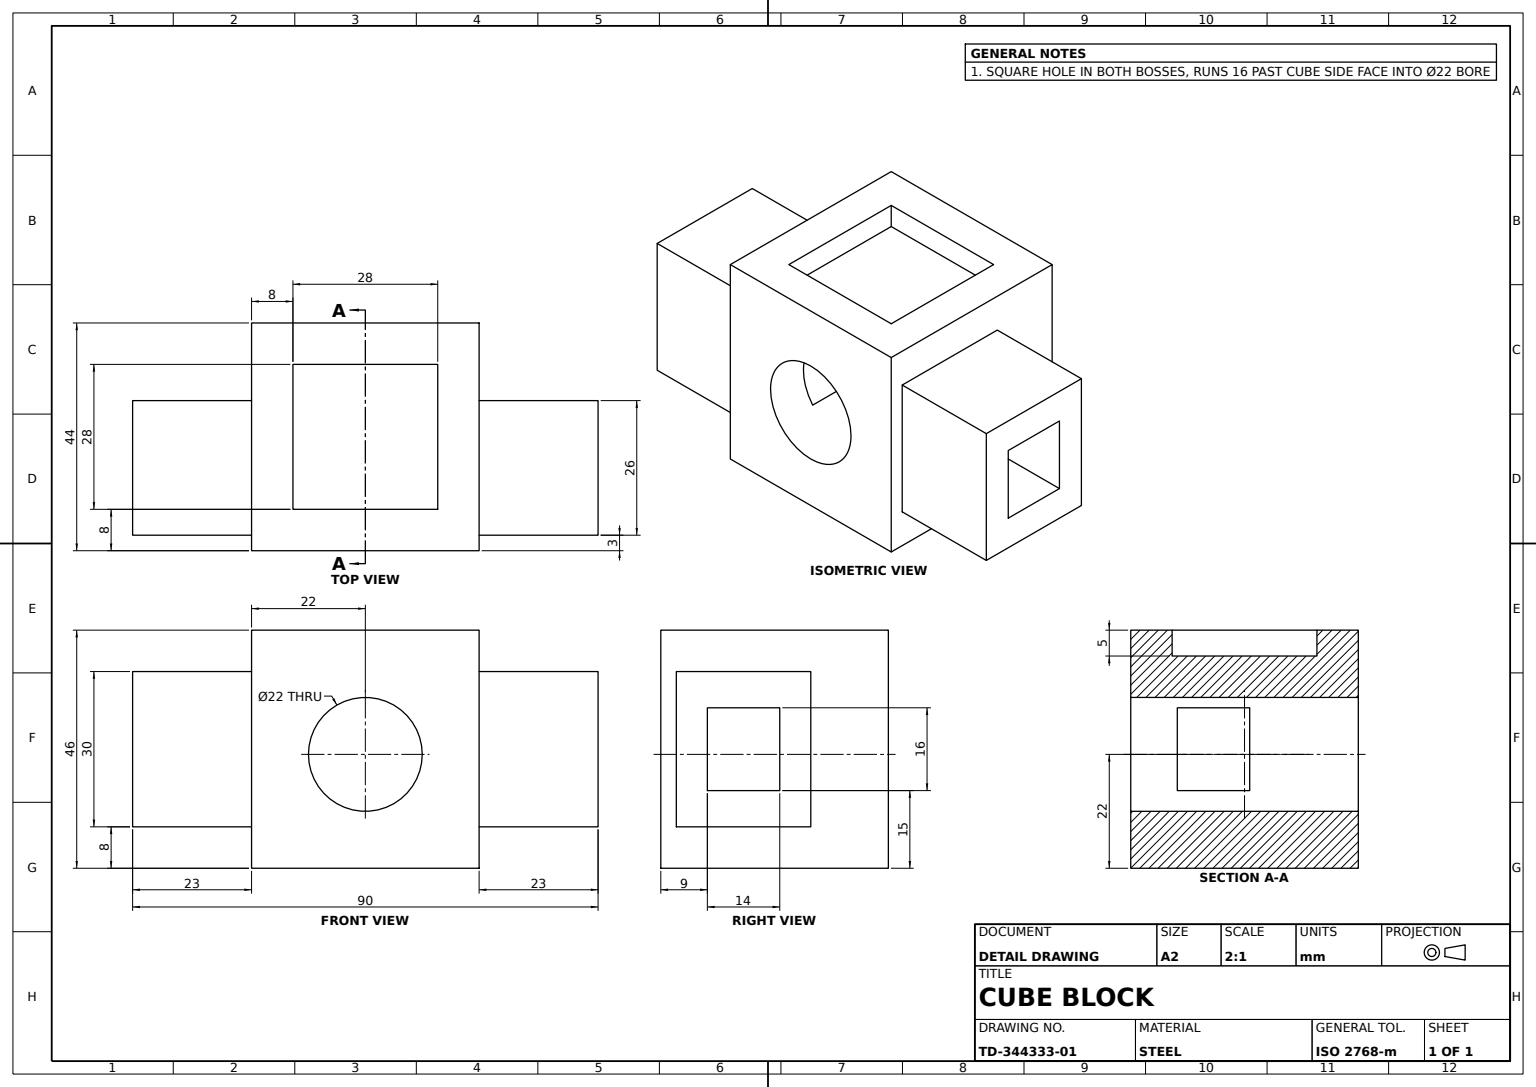
SolidWorks part; units mm, degrees
material "Plain Carbon Steel"
ref_plane "Front Plane" through (0, 0, 0) normal (0, 0, 1) x (1, 0, 0)
ref_plane "Top Plane" through (0, 0, 0) normal (0, 1, 0) x (1, 0, 0)
ref_plane "Right Plane" through (0, 0, 0) normal (1, 0, 0) x (0, 0, -1)
sketch "Main Block Profile" plane through (0, 0, 0) normal (0, 0, 1) x (1, 0, 0)
  line L1 (-22, -23) -> (22, -23)
  line L2 (-22, -23) -> (-22, 23)
  line L3 (-22, 23) -> (22, 23)
  line L4 (22, -23) -> (22, 23)
  line L5 (-22, -23) -> (22, 23) construction
  line L6 (-22, 23) -> (22, -23) construction
  circle A0 centre (0, -1) radius 11
  point P0 (0, 0)
  dimension "D3" = 22
  dimension "D1" = 44
  dimension "D2" = 46
  dimension "D4" = 22
extrude "Main Block 44mm" add sketch "Main Block Profile" against normal blind 44
sketch "Top Pocket Profile 28x28" plane through (0, 23, 0) normal (0, 1, 0) x (1, 0, 0)
  line L0 (22, 44) -> (-22, 44) construction
  line L1 (-14, 8) -> (14, 8)
  line L2 (-14, 8) -> (-14, 36)
  line L3 (-14, 36) -> (14, 36)
  line L4 (14, 8) -> (14, 36)
  line L5 (-14, 8) -> (14, 36) construction
  line L6 (-14, 36) -> (14, 8) construction
  line L7 (22, 44) -> (22, 0) construction
  point P0 (0, 22)
  dimension "D1" = 28
  dimension "D2" = 28
  dimension "D3" = 8
  dimension "D4" = 8
extrude "Top Square Pocket 28x28x5" cut sketch "Top Pocket Profile 28x28" against normal blind 5
sketch "Side Boss Profile" plane through (-22, 0, 0) normal (-1, 0, 0) x (0, 0, 1)
  line L0 (-44, 23) -> (-44, -23) construction
  line L1 (-29, 15) -> (-3, 15)
  line L2 (-29, 15) -> (-29, -15)
  line L3 (-29, -15) -> (-3, -15)
  line L4 (-3, 15) -> (-3, -15)
  line L5 (-29, 15) -> (-3, -15) construction
  line L6 (-29, -15) -> (-3, 15) construction
  line L7 (-23, 8) -> (-9, 8)
  line L8 (-23, 8) -> (-23, -8)
  line L9 (-23, -8) -> (-9, -8)
  line L10 (-9, 8) -> (-9, -8)
  line L11 (-23, 8) -> (-9, -8) construction
  line L12 (-23, -8) -> (-9, 8) construction
  line L14 (-44, 23) -> (0, 23) construction
  point P0 (-16, 0)
  point P5 (-16, 0)
  dimension "D1" = 30
  dimension "D2" = 26
  dimension "D3" = 15
  dimension "D4" = 14
  dimension "D5" = 16
  dimension "D6" = 8
extrude "Side Square Boss 23mm" add sketch "Side Boss Profile" along normal blind 23
mirror "Side Boss Mirror" about plane through (0, 0, 0) normal (1, 0, 0) of "Side Square Boss 23mm"
sketch "Side Opening Profile" plane through (45, 0, 0) normal (1, 0, 0) x (0, 0, -1)
  line L0 (9, -8) -> (9, 8)
  line L1 (9, -8) -> (9, 8) construction
  line L2 (9, -8) -> (9, 8) construction
  line L3 (9, 8) -> (23, 8)
  line L4 (23, 8) -> (23, -8)
  line L5 (23, -8) -> (9, -8)
extrude "Side Opening Cut" cut sketch "Side Opening Profile" against normal through all
